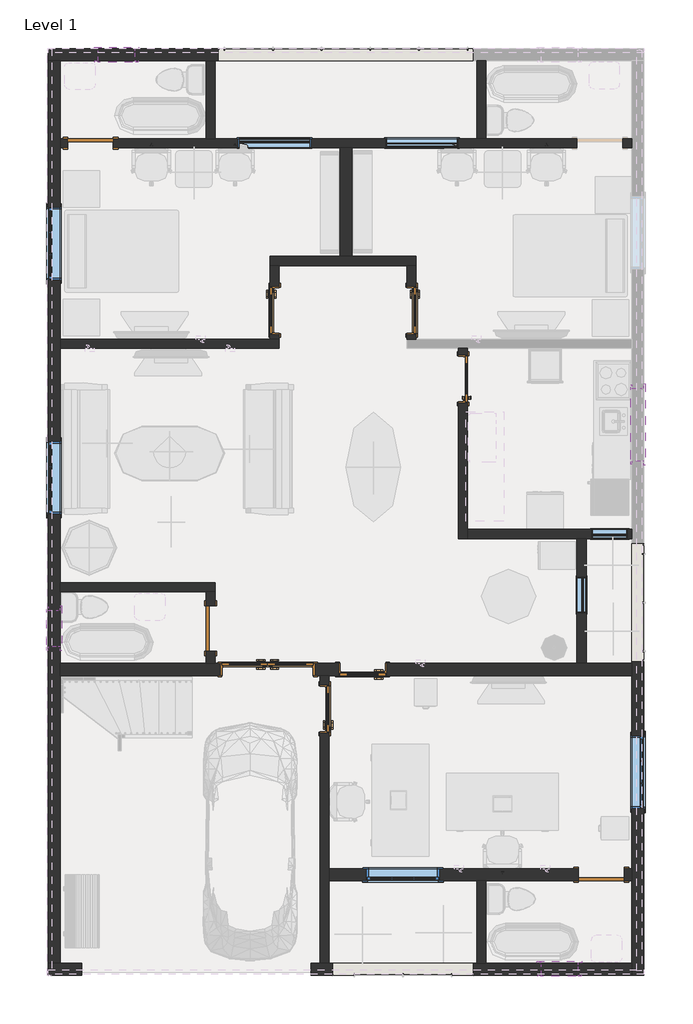
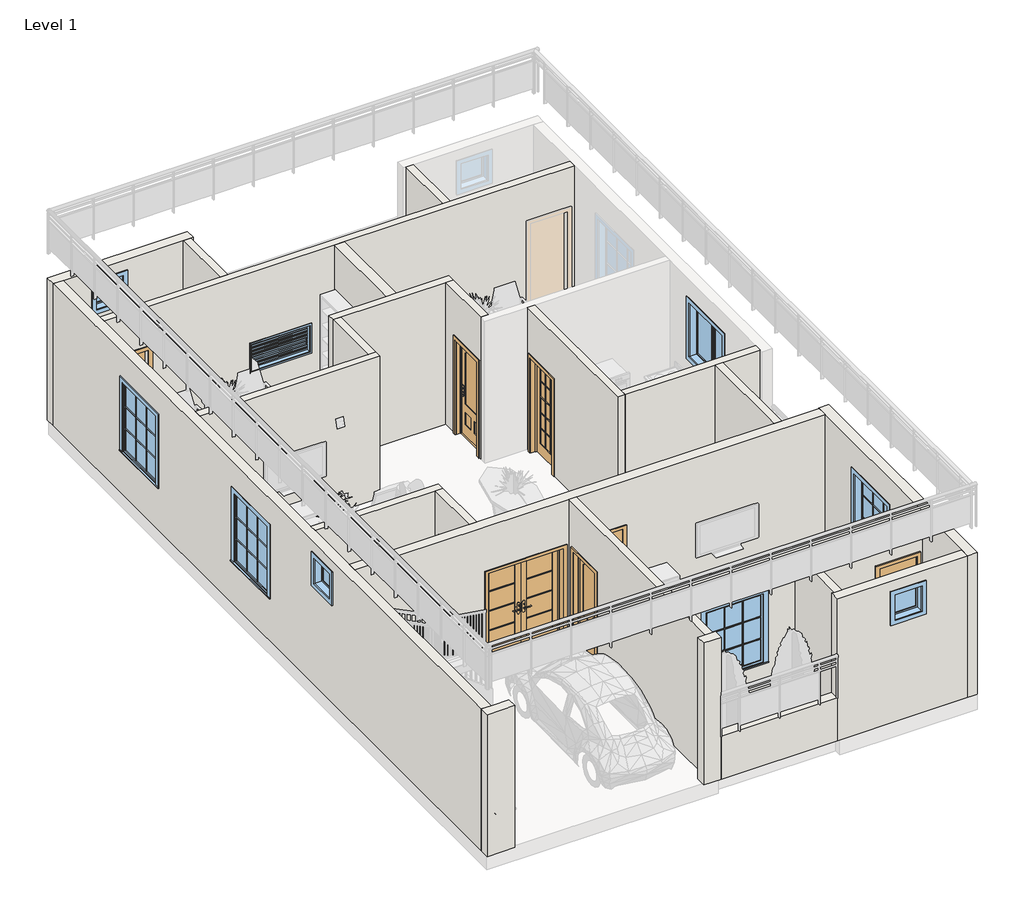
# One storey, part 1 of 5: 26 walls, 12 windows, 9 doors.
"""IFC4 building model written with IfcOpenShell, lengths in millimetres."""

from ifc_helpers import new_model, si_unit, frame, origin, origin_with_axes, place, context, project, spatial, polyline, outline, extrude, faceted_brep, transform, mapped, element, save
from components import door_14b9be53, door_41326d50, door_4b146b56, door_b03bd389, door_a0b5ff2a, door_e2b13fe9, door_4314e8ec, window_cfa1ffdd, window_0862ab64, window_67e7833d, louvers_with_trim_double_60c1390f, window_e41d21a6

model = new_model("IFC4")

# Units and contexts
model_context = context("Model", 3, world=origin())
ifc_project = project(units=[si_unit("LENGTHUNIT", "METRE", prefix="MILLI")], contexts=[model_context])

# Site, building, storey
site = spatial("IfcSite", under=ifc_project)
building = spatial("IfcBuilding", under=site)
storey = spatial("IfcBuildingStorey", under=building, Name="Level 1", Elevation=0.0)

# Doors
placement = place(None, origin())
door_shape = door_14b9be53(model_context)
element("IfcDoor", 1, ObjectType="30\" x 80\"", at=placement, inside=storey, context=model_context, shape_type="MappedRepresentation", body=[
    mapped(door_shape, transform((-2673.2207152, 5044.1691167, 0.0), x_axis=(0.0, -1.0, 0.0), y_axis=(1.0, 0.0, 0.0), z_axis=(0.0, 0.0, 1.0))),
])
element("IfcDoor", 2, ObjectType="30\" x 80\"", at=placement, inside=storey, context=model_context, shape_type="MappedRepresentation", body=[
    mapped(door_shape, transform((-3514.5967824, 11698.9691167, 0.0), x_axis=(0.0, 1.0, 0.0), y_axis=(-1.0, 0.0, 0.0), z_axis=(0.0, 0.0, 1.0))),
])
door_2_shape = door_41326d50(model_context)
element("IfcDoor", 3, ObjectType="30\" x 80\"", at=placement, inside=storey, context=model_context, shape_type="MappedRepresentation", body=[
    mapped(door_2_shape, transform((-2041.3957152, 5701.3941167, 0.0), x_axis=(1.0, 0.0, 0.0), y_axis=(0.0, 1.0, 0.0), z_axis=(0.0, 0.0, 1.0))),
])
door_3_shape = door_4b146b56(model_context)
element("IfcDoor", 4, ObjectType="30\" x 80\"", at=placement, inside=storey, context=model_context, shape_type="MappedRepresentation", body=[
    mapped(door_3_shape, transform((-1222.2467824, 11698.9691167, 0.0), x_axis=(0.0, 1.0, 0.0), y_axis=(-1.0, 0.0, 0.0), z_axis=(0.0, 0.0, 1.0))),
])
door_4_shape = door_b03bd389(model_context)
element("IfcDoor", 5, ObjectType="Door-Exterior-Double-Full Glass-Wood_Clad : 60\" x 80\"", at=placement, inside=storey, context=model_context, shape_type="MappedRepresentation", body=[
    mapped(door_4_shape, transform((-3628.8957152, 5707.7441167, 0.0), x_axis=(1.0, 0.0, 0.0), y_axis=(0.0, 1.0, 0.0), z_axis=(0.0, 0.0, 1.0))),
])
door_5_shape = door_a0b5ff2a(model_context)
element("IfcDoor", 6, ObjectType="Door-Interior-Single-Full Glass-Wood : 30\" x 80\"", at=placement, inside=storey, context=model_context, shape_type="MappedRepresentation", body=[
    mapped(door_5_shape, transform((-361.8207152, 10555.9691167, 0.0), x_axis=(0.0, 1.0, 0.0), y_axis=(-1.0, 0.0, 0.0), z_axis=(0.0, 0.0, 1.0))),
])
door_6_shape = door_e2b13fe9(model_context)
element("IfcDoor", 7, ObjectType="Single-Flush : 30\" x 84\"", at=placement, inside=storey, context=model_context, shape_type="MappedRepresentation", body=[
    mapped(door_6_shape, transform((-6587.9957152, 14492.9691167, 0.0), x_axis=(-1.0, 0.0, 0.0), y_axis=(0.0, -1.0, 0.0), z_axis=(0.0, 0.0, 1.0))),
])
element("IfcDoor", 8, ObjectType="Single-Flush : 30\" x 84\"", at=placement, inside=storey, context=model_context, shape_type="MappedRepresentation", body=[
    mapped(door_6_shape, transform((-4581.3957152, 6390.3691167, 0.0), x_axis=(0.0, -1.0, 0.0), y_axis=(1.0, 0.0, 0.0), z_axis=(0.0, 0.0, 1.0))),
])
door_7_shape = door_4314e8ec(model_context)
element("IfcDoor", 9, ObjectType="Single-Flush : 30\" x 84\"", at=placement, inside=storey, context=model_context, shape_type="MappedRepresentation", body=[
    mapped(door_7_shape, transform((1946.4042848, 2275.5691167, 0.0), x_axis=(1.0, 0.0, 0.0), y_axis=(0.0, 1.0, 0.0), z_axis=(0.0, 0.0, 1.0))),
])

# Walls
element("IfcWall", 10, ObjectType="Generic - 8\"", at=placement, inside=storey, context=model_context, shape_type="Brep", body=[
    faceted_brep([(-7299.1957152, 15864.5691167, 0.0), (-7095.9957152, 15864.5691167, 0.0), (-4657.5957152, 15864.5691167, 0.0), (-4505.1957152, 15864.5691167, 0.0), (-4454.3957152, 15864.5691167, 0.0), (-4454.3957152, 15864.5691167, 914.4), (-4454.3957152, 15864.5691167, 3048.0), (-4505.1957152, 15864.5691167, 3048.0), (-4657.5957152, 15864.5691167, 3048.0), (-7095.9957152, 15864.5691167, 3048.0), (-7299.1957152, 15864.5691167, 3048.0), (-5851.3957152, 15864.5691167, 2768.6), (-5851.3957152, 15864.5691167, 2159.0), (-6460.9957152, 15864.5691167, 2159.0), (-6460.9957152, 15864.5691167, 2768.6), (-7299.1957152, 16067.7691167, 0.0), (-7299.1957152, 16067.7691167, 3048.0), (-4454.3957152, 16067.7691167, 3048.0), (-4454.3957152, 16067.7691167, 914.4), (-4454.3957152, 16067.7691167, 0.0), (-5851.3957152, 16067.7691167, 2768.6), (-6460.9957152, 16067.7691167, 2768.6), (-6460.9957152, 16067.7691167, 2159.0), (-5851.3957152, 16067.7691167, 2159.0)], [[[0, 1, 2, 3, 4, 5, 6, 7, 8, 9, 10], [11, 12, 13, 14]], [[15, 16, 17, 18, 19], [20, 21, 22, 23]], [[4, 3, 2, 1, 0, 15, 19]], [[6, 5, 4, 19, 18, 17]], [[0, 10, 16, 15]], [[10, 9, 8, 7, 6, 17, 16]], [[12, 11, 20, 23]], [[13, 12, 23, 22]], [[14, 13, 22, 21]], [[11, 14, 21, 20]]]),
])
element("IfcWall", 11, ObjectType="Generic - 8\"", at=placement, inside=storey, context=model_context, shape_type="Brep", body=[
    faceted_brep([(2454.4042848, 802.3691167, 0.0), (16.0042848, 802.3691167, 0.0), (-136.3957152, 802.3691167, 0.0), (-187.1957152, 802.3691167, 0.0), (-187.1957152, 802.3691167, 914.4), (-187.1957152, 802.3691167, 3048.0), (-136.3957152, 802.3691167, 3048.0), (16.0042848, 802.3691167, 3048.0), (2454.4042848, 802.3691167, 3048.0), (1552.7042848, 802.3691167, 2768.6), (943.1042848, 802.3691167, 2768.6), (943.1042848, 802.3691167, 2159.0), (1552.7042848, 802.3691167, 2159.0), (2454.4042848, 599.1691167, 0.0), (2454.4042848, 599.1691167, 3048.0), (-187.1957152, 599.1691167, 3048.0), (-187.1957152, 599.1691167, 914.4), (-187.1957152, 599.1691167, 0.0), (1552.7042848, 599.1691167, 2768.6), (1552.7042848, 599.1691167, 2159.0), (943.1042848, 599.1691167, 2159.0), (943.1042848, 599.1691167, 2768.6)], [[[0, 1, 2, 3, 4, 5, 6, 7, 8], [9, 10, 11, 12]], [[13, 14, 15, 16, 17], [18, 19, 20, 21]], [[3, 2, 1, 0, 13, 17]], [[5, 4, 3, 17, 16, 15]], [[0, 8, 14, 13]], [[8, 7, 6, 5, 15, 14]], [[19, 18, 9, 12]], [[20, 19, 12, 11]], [[21, 20, 11, 10]], [[18, 21, 10, 9]]]),
])
element("IfcWall", 12, ObjectType="Generic - 8\"", at=placement, inside=storey, context=model_context, shape_type="Brep", body=[
    faceted_brep([(-7095.9957152, 802.3691167, 0.0), (-7095.9957152, 5602.9691167, 0.0), (-7095.9957152, 5806.1691167, 0.0), (-7095.9957152, 6999.9691167, 0.0), (-7095.9957152, 7152.3691167, 0.0), (-7095.9957152, 11063.9691167, 0.0), (-7095.9957152, 11216.3691167, 0.0), (-7095.9957152, 14416.7691167, 0.0), (-7095.9957152, 14569.1691167, 0.0), (-7095.9957152, 15864.5691167, 0.0), (-7095.9957152, 15864.5691167, 3048.0), (-7095.9957152, 14569.1691167, 3048.0), (-7095.9957152, 14416.7691167, 3048.0), (-7095.9957152, 11216.3691167, 3048.0), (-7095.9957152, 11063.9691167, 3048.0), (-7095.9957152, 7152.3691167, 3048.0), (-7095.9957152, 6999.9691167, 3048.0), (-7095.9957152, 5806.1691167, 3048.0), (-7095.9957152, 5602.9691167, 3048.0), (-7095.9957152, 802.3691167, 3048.0), (-7095.9957152, 9514.5691167, 2438.4), (-7095.9957152, 9514.5691167, 914.4), (-7095.9957152, 8295.3691167, 914.4), (-7095.9957152, 8295.3691167, 2438.4), (-7095.9957152, 13426.1691167, 2438.4), (-7095.9957152, 13426.1691167, 914.4), (-7095.9957152, 12206.9691167, 914.4), (-7095.9957152, 12206.9691167, 2438.4), (-7095.9957152, 6085.5691167, 2768.6), (-7095.9957152, 6695.1691167, 2768.6), (-7095.9957152, 6695.1691167, 2159.0), (-7095.9957152, 6085.5691167, 2159.0), (-7299.1957152, 802.3691167, 0.0), (-7299.1957152, 802.3691167, 3048.0), (-7299.1957152, 15864.5691167, 3048.0), (-7299.1957152, 15864.5691167, 0.0), (-7299.1957152, 9514.5691167, 2438.4), (-7299.1957152, 8295.3691167, 2438.4), (-7299.1957152, 8295.3691167, 914.4), (-7299.1957152, 9514.5691167, 914.4), (-7299.1957152, 13426.1691167, 2438.4), (-7299.1957152, 12206.9691167, 2438.4), (-7299.1957152, 12206.9691167, 914.4), (-7299.1957152, 13426.1691167, 914.4), (-7299.1957152, 6085.5691167, 2768.6), (-7299.1957152, 6085.5691167, 2159.0), (-7299.1957152, 6695.1691167, 2159.0), (-7299.1957152, 6695.1691167, 2768.6)], [[[0, 1, 2, 3, 4, 5, 6, 7, 8, 9, 10, 11, 12, 13, 14, 15, 16, 17, 18, 19], [20, 21, 22, 23], [24, 25, 26, 27], [28, 29, 30, 31]], [[32, 33, 34, 35], [36, 37, 38, 39], [40, 41, 42, 43], [44, 45, 46, 47]], [[9, 8, 7, 6, 5, 4, 3, 2, 1, 0, 32, 35]], [[10, 9, 35, 34]], [[0, 19, 33, 32]], [[19, 18, 17, 16, 15, 14, 13, 12, 11, 10, 34, 33]], [[21, 20, 36, 39]], [[22, 21, 39, 38]], [[23, 22, 38, 37]], [[20, 23, 37, 36]], [[25, 24, 40, 43]], [[26, 25, 43, 42]], [[27, 26, 42, 41]], [[24, 27, 41, 40]], [[45, 44, 28, 31]], [[46, 45, 31, 30]], [[47, 46, 30, 29]], [[44, 47, 29, 28]]]),
])
element("IfcWall", 13, ObjectType="Generic - 8\"", at=placement, inside=storey, context=model_context, shape_type="Brep", body=[
    faceted_brep([(2454.4042848, 5602.9691167, 0.0), (2454.4042848, 5602.9691167, 3048.0), (-2600.1957152, 5602.9691167, 3048.0), (-2752.5957152, 5602.9691167, 3048.0), (-7095.9957152, 5602.9691167, 3048.0), (-7095.9957152, 5602.9691167, 0.0), (-4416.2957152, 5602.9691167, 0.0), (-4416.2957152, 5602.9691167, 2057.4), (-2841.4957152, 5602.9691167, 2057.4), (-2841.4957152, 5602.9691167, 0.0), (-2752.5957152, 5602.9691167, 0.0), (-2600.1957152, 5602.9691167, 0.0), (-2447.7957152, 5602.9691167, 0.0), (-2447.7957152, 5602.9691167, 2057.4), (-1634.9957152, 5602.9691167, 2057.4), (-1634.9957152, 5602.9691167, 0.0), (-7095.9957152, 5806.1691167, 3048.0), (-4657.5957152, 5806.1691167, 3048.0), (-4505.1957152, 5806.1691167, 3048.0), (1540.0042848, 5806.1691167, 3048.0), (1692.4042848, 5806.1691167, 3048.0), (2454.4042848, 5806.1691167, 3048.0), (2454.4042848, 5806.1691167, 0.0), (1692.4042848, 5806.1691167, 0.0), (1540.0042848, 5806.1691167, 0.0), (-1634.9957152, 5806.1691167, 0.0), (-1634.9957152, 5806.1691167, 2057.4), (-2447.7957152, 5806.1691167, 2057.4), (-2447.7957152, 5806.1691167, 0.0), (-2841.4957152, 5806.1691167, 0.0), (-2841.4957152, 5806.1691167, 2057.4), (-4416.2957152, 5806.1691167, 2057.4), (-4416.2957152, 5806.1691167, 0.0), (-4505.1957152, 5806.1691167, 0.0), (-4657.5957152, 5806.1691167, 0.0), (-7095.9957152, 5806.1691167, 0.0)], [[[0, 1, 2, 3, 4, 5, 6, 7, 8, 9, 10, 11, 12, 13, 14, 15]], [[16, 17, 18, 19, 20, 21, 22, 23, 24, 25, 26, 27, 28, 29, 30, 31, 32, 33, 34, 35]], [[5, 35, 34, 33, 32, 6]], [[22, 0, 15, 25, 24, 23]], [[9, 29, 28, 12, 11, 10]], [[1, 0, 22, 21]], [[5, 4, 16, 35]], [[21, 20, 19, 18, 17, 16, 4, 3, 2, 1]], [[8, 30, 29, 9]], [[30, 8, 7, 31]], [[31, 7, 6, 32]], [[14, 26, 25, 15]], [[26, 14, 13, 27]], [[27, 13, 12, 28]]]),
])
element("IfcWall", 14, ObjectType="Generic - 8\"", at=placement, inside=storey, context=model_context, shape_type="Brep", body=[
    faceted_brep([(2327.4042848, 2173.9691167, 2133.6), (2327.4042848, 2173.9691167, 0.0), (2454.4042848, 2173.9691167, 0.0), (2454.4042848, 2173.9691167, 3048.0), (16.0042848, 2173.9691167, 3048.0), (-136.3957152, 2173.9691167, 3048.0), (-2600.1957152, 2173.9691167, 3048.0), (-2600.1957152, 2173.9691167, 0.0), (-136.3957152, 2173.9691167, 0.0), (16.0042848, 2173.9691167, 0.0), (1565.4042848, 2173.9691167, 0.0), (1565.4042848, 2173.9691167, 2133.6), (-1977.8957152, 2173.9691167, 2438.4), (-758.6957152, 2173.9691167, 2438.4), (-758.6957152, 2173.9691167, 914.4), (-1977.8957152, 2173.9691167, 914.4), (2454.4042848, 2377.1691167, 0.0), (2327.4042848, 2377.1691167, 0.0), (2327.4042848, 2377.1691167, 2133.6), (1565.4042848, 2377.1691167, 2133.6), (1565.4042848, 2377.1691167, 0.0), (-2600.1957152, 2377.1691167, 0.0), (-2600.1957152, 2377.1691167, 3048.0), (2454.4042848, 2377.1691167, 3048.0), (-1977.8957152, 2377.1691167, 2438.4), (-1977.8957152, 2377.1691167, 914.4), (-758.6957152, 2377.1691167, 914.4), (-758.6957152, 2377.1691167, 2438.4)], [[[0, 1, 2, 3, 4, 5, 6, 7, 8, 9, 10, 11], [12, 13, 14, 15]], [[16, 17, 18, 19, 20, 21, 22, 23], [24, 25, 26, 27]], [[2, 1, 17, 16]], [[10, 9, 8, 7, 21, 20]], [[3, 2, 16, 23]], [[7, 6, 22, 21]], [[6, 5, 4, 3, 23, 22]], [[18, 17, 1, 0]], [[19, 18, 0, 11]], [[20, 19, 11, 10]], [[25, 24, 12, 15]], [[26, 25, 15, 14]], [[27, 26, 14, 13]], [[24, 27, 13, 12]]]),
])
element("IfcWall", 15, ObjectType="Generic - 8\"", at=placement, inside=storey, context=model_context, shape_type="SweptSolid", body=[
    extrude(outline(polyline([(-2422.3957152, 12601.2939646), (-2422.3957152, 14416.7691167), (-2219.1957152, 14416.7691167), (-2219.1957152, 12601.2939646), (-2422.3957152, 12601.2939646)])), origin_with_axes(), (0.0, 0.0, 1.0), 3048.0),
])
element("IfcWall", 16, ObjectType="Generic - 8\"", at=placement, inside=storey, context=model_context, shape_type="SweptSolid", body=[
    extrude(outline(polyline([(-187.1957152, 15864.5691167), (-4454.3957152, 15864.5691167), (-4454.3957152, 16067.7691167), (-187.1957152, 16067.7691167), (-187.1957152, 15864.5691167)])), origin_with_axes(), (0.0, 0.0, 1.0), 914.4),
])
element("IfcWall", 17, ObjectType="Generic - 8\"", at=placement, inside=storey, context=model_context, shape_type="SweptSolid", body=[
    extrude(outline(polyline([(2454.4042848, 5831.5691167), (2454.4042848, 7812.7691167), (2657.6042848, 7812.7691167), (2657.6042848, 5831.5691167), (2454.4042848, 5831.5691167)])), origin_with_axes(), (0.0, 0.0, 1.0), 914.4),
])
element("IfcWall", 18, ObjectType="Generic - 8\"", at=placement, inside=storey, context=model_context, shape_type="Brep", body=[
    faceted_brep([(2454.4042848, 5831.5691167, 0.0), (2454.4042848, 5806.1691167, 0.0), (2454.4042848, 5602.9691167, 0.0), (2454.4042848, 2377.1691167, 0.0), (2454.4042848, 2173.9691167, 0.0), (2454.4042848, 802.3691167, 0.0), (2454.4042848, 599.1691167, 0.0), (2454.4042848, 599.1691167, 3048.0), (2454.4042848, 802.3691167, 3048.0), (2454.4042848, 2173.9691167, 3048.0), (2454.4042848, 2377.1691167, 3048.0), (2454.4042848, 5602.9691167, 3048.0), (2454.4042848, 5806.1691167, 3048.0), (2454.4042848, 5831.5691167, 3048.0), (2454.4042848, 5831.5691167, 914.4), (2454.4042848, 3380.4691167, 2438.4), (2454.4042848, 3380.4691167, 914.4), (2454.4042848, 4599.6691167, 914.4), (2454.4042848, 4599.6691167, 2438.4), (2657.6042848, 5831.5691167, 0.0), (2657.6042848, 5831.5691167, 914.4), (2657.6042848, 5831.5691167, 3048.0), (2657.6042848, 599.1691167, 3048.0), (2657.6042848, 599.1691167, 0.0), (2657.6042848, 3380.4691167, 2438.4), (2657.6042848, 4599.6691167, 2438.4), (2657.6042848, 4599.6691167, 914.4), (2657.6042848, 3380.4691167, 914.4)], [[[0, 1, 2, 3, 4, 5, 6, 7, 8, 9, 10, 11, 12, 13, 14], [15, 16, 17, 18]], [[19, 20, 21, 22, 23], [24, 25, 26, 27]], [[6, 5, 4, 3, 2, 1, 0, 19, 23]], [[0, 14, 13, 21, 20, 19]], [[7, 6, 23, 22]], [[13, 12, 11, 10, 9, 8, 7, 22, 21]], [[16, 15, 24, 27]], [[17, 16, 27, 26]], [[18, 17, 26, 25]], [[15, 18, 25, 24]]]),
])
element("IfcWall", 19, ObjectType="Generic - 8\"", at=placement, inside=storey, context=model_context, shape_type="Brep", body=[
    faceted_brep([(-6740.3957152, 802.3691167, 0.0), (-7095.9957152, 802.3691167, 0.0), (-7299.1957152, 802.3691167, 0.0), (-7299.1957152, 802.3691167, 3048.0), (-7095.9957152, 802.3691167, 3048.0), (-6740.3957152, 802.3691167, 3048.0), (-6740.3957152, 599.1691167, 0.0), (-6740.3957152, 599.1691167, 3048.0), (-7299.1957152, 599.1691167, 3048.0), (-7299.1957152, 599.1691167, 0.0)], [[[0, 1, 2, 3, 4, 5]], [[6, 7, 8, 9]], [[2, 1, 0, 6, 9]], [[0, 5, 7, 6]], [[3, 2, 9, 8]], [[5, 4, 3, 8, 7]]]),
])
element("IfcWall", 20, ObjectType="Generic - 8\"", at=placement, inside=storey, context=model_context, shape_type="Brep", body=[
    faceted_brep([(-2549.3957152, 802.3691167, 0.0), (-2600.1957152, 802.3691167, 0.0), (-2752.5957152, 802.3691167, 0.0), (-2904.9957152, 802.3691167, 0.0), (-2904.9957152, 802.3691167, 3048.0), (-2752.5957152, 802.3691167, 3048.0), (-2600.1957152, 802.3691167, 3048.0), (-2549.3957152, 802.3691167, 3048.0), (-2549.3957152, 802.3691167, 914.4), (-2549.3957152, 599.1691167, 0.0), (-2549.3957152, 599.1691167, 914.4), (-2549.3957152, 599.1691167, 3048.0), (-2904.9957152, 599.1691167, 3048.0), (-2904.9957152, 599.1691167, 0.0)], [[[0, 1, 2, 3, 4, 5, 6, 7, 8]], [[9, 10, 11, 12, 13]], [[3, 2, 1, 0, 9, 13]], [[4, 3, 13, 12]], [[0, 8, 7, 11, 10, 9]], [[7, 6, 5, 4, 12, 11]]]),
])
element("IfcWall", 21, ObjectType="Generic - 8\"", at=placement, inside=storey, context=model_context, shape_type="SweptSolid", body=[
    extrude(outline(polyline([(-2549.3957152, 802.3691167), (-187.1957152, 802.3691167), (-187.1957152, 599.1691167), (-2549.3957152, 599.1691167), (-2549.3957152, 802.3691167)])), origin_with_axes(), (0.0, 0.0, 1.0), 914.4),
])
element("IfcWall", 22, ObjectType="inner wall", at=placement, inside=storey, context=model_context, shape_type="Brep", body=[
    faceted_brep([(2302.0042848, 14416.7691167, 2133.6), (2302.0042848, 14416.7691167, 0.0), (2454.4042848, 14416.7691167, 0.0), (2454.4042848, 14416.7691167, 3048.0), (-2219.1957152, 14416.7691167, 3048.0), (-2422.3957152, 14416.7691167, 3048.0), (-7095.9957152, 14416.7691167, 3048.0), (-7095.9957152, 14416.7691167, 0.0), (-6968.9957152, 14416.7691167, 0.0), (-6968.9957152, 14416.7691167, 2133.6), (-6206.9957152, 14416.7691167, 2133.6), (-6206.9957152, 14416.7691167, 0.0), (-2422.3957152, 14416.7691167, 0.0), (-2219.1957152, 14416.7691167, 0.0), (1540.0042848, 14416.7691167, 0.0), (1540.0042848, 14416.7691167, 2133.6), (-2904.9957152, 14416.7691167, 1524.0), (-2904.9957152, 14416.7691167, 914.4), (-4124.1957152, 14416.7691167, 914.4), (-4124.1957152, 14416.7691167, 1524.0), (-1660.3957152, 14416.7691167, 1524.0), (-441.1957152, 14416.7691167, 1524.0), (-441.1957152, 14416.7691167, 914.4), (-1660.3957152, 14416.7691167, 914.4), (2454.4042848, 14569.1691167, 0.0), (2302.0042848, 14569.1691167, 0.0), (2302.0042848, 14569.1691167, 2133.6), (1540.0042848, 14569.1691167, 2133.6), (1540.0042848, 14569.1691167, 0.0), (16.0042848, 14569.1691167, 0.0), (-136.3957152, 14569.1691167, 0.0), (-4505.1957152, 14569.1691167, 0.0), (-4657.5957152, 14569.1691167, 0.0), (-6206.9957152, 14569.1691167, 0.0), (-6206.9957152, 14569.1691167, 2133.6), (-6968.9957152, 14569.1691167, 2133.6), (-6968.9957152, 14569.1691167, 0.0), (-7095.9957152, 14569.1691167, 0.0), (-7095.9957152, 14569.1691167, 3048.0), (-4657.5957152, 14569.1691167, 3048.0), (-4505.1957152, 14569.1691167, 3048.0), (-136.3957152, 14569.1691167, 3048.0), (16.0042848, 14569.1691167, 3048.0), (2454.4042848, 14569.1691167, 3048.0), (-2904.9957152, 14569.1691167, 1524.0), (-4124.1957152, 14569.1691167, 1524.0), (-4124.1957152, 14569.1691167, 914.4), (-2904.9957152, 14569.1691167, 914.4), (-1660.3957152, 14569.1691167, 1524.0), (-1660.3957152, 14569.1691167, 914.4), (-441.1957152, 14569.1691167, 914.4), (-441.1957152, 14569.1691167, 1524.0)], [[[0, 1, 2, 3, 4, 5, 6, 7, 8, 9, 10, 11, 12, 13, 14, 15], [16, 17, 18, 19], [20, 21, 22, 23]], [[24, 25, 26, 27, 28, 29, 30, 31, 32, 33, 34, 35, 36, 37, 38, 39, 40, 41, 42, 43], [44, 45, 46, 47], [48, 49, 50, 51]], [[37, 36, 8, 7]], [[2, 1, 25, 24]], [[14, 13, 12, 11, 33, 32, 31, 30, 29, 28]], [[3, 2, 24, 43]], [[7, 6, 38, 37]], [[6, 5, 4, 3, 43, 42, 41, 40, 39, 38]], [[9, 8, 36, 35]], [[10, 9, 35, 34]], [[11, 10, 34, 33]], [[26, 25, 1, 0]], [[27, 26, 0, 15]], [[28, 27, 15, 14]], [[17, 16, 44, 47]], [[18, 17, 47, 46]], [[19, 18, 46, 45]], [[16, 19, 45, 44]], [[49, 48, 20, 23]], [[50, 49, 23, 22]], [[51, 50, 22, 21]], [[48, 51, 21, 20]]]),
])
element("IfcWall", 23, ObjectType="inner wall", at=placement, inside=storey, context=model_context, shape_type="SweptSolid", body=[
    extrude(outline(polyline([(-4657.5957152, 14569.1691167), (-4657.5957152, 15864.5691167), (-4505.1957152, 15864.5691167), (-4505.1957152, 14569.1691167), (-4657.5957152, 14569.1691167)])), origin_with_axes(), (0.0, 0.0, 1.0), 3048.0),
])
element("IfcWall", 24, ObjectType="inner wall", at=placement, inside=storey, context=model_context, shape_type="SweptSolid", body=[
    extrude(outline(polyline([(-136.3957152, 14569.1691167), (-136.3957152, 15864.5691167), (16.0042848, 15864.5691167), (16.0042848, 14569.1691167), (-136.3957152, 14569.1691167)])), origin_with_axes(), (0.0, 0.0, 1.0), 3048.0),
])
element("IfcWall", 25, ObjectType="inner wall", at=placement, inside=storey, context=model_context, shape_type="Brep", body=[
    faceted_brep([(-7095.9957152, 11063.9691167, 0.0), (-3435.2217824, 11063.9691167, 0.0), (-3435.2217824, 11063.9691167, 3048.0), (-7095.9957152, 11063.9691167, 3048.0), (-7095.9957152, 11216.3691167, 0.0), (-7095.9957152, 11216.3691167, 3048.0), (-3587.6217824, 11216.3691167, 3048.0), (-3435.2217824, 11216.3691167, 3048.0), (-3435.2217824, 11216.3691167, 0.0), (-3587.6217824, 11216.3691167, 0.0)], [[[0, 1, 2, 3]], [[4, 5, 6, 7, 8, 9]], [[1, 0, 4, 9, 8]], [[0, 3, 5, 4]], [[2, 1, 8, 7]], [[3, 2, 7, 6, 5]]]),
])
element("IfcWall", 26, ObjectType="inner wall", at=placement, inside=storey, context=model_context, shape_type="Brep", body=[
    faceted_brep([(-2752.5957152, 802.3691167, 0.0), (-2752.5957152, 802.3691167, 3048.0), (-2752.5957152, 3036.4892317, 3048.0), (-2752.5957152, 5602.9691167, 3048.0), (-2752.5957152, 5602.9691167, 0.0), (-2752.5957152, 5450.5691167, 0.0), (-2752.5957152, 5450.5691167, 2057.4), (-2752.5957152, 4637.7691167, 2057.4), (-2752.5957152, 4637.7691167, 0.0), (-2600.1957152, 5602.9691167, 3048.0), (-2600.1957152, 2377.1691167, 3048.0), (-2600.1957152, 2173.9691167, 3048.0), (-2600.1957152, 802.3691167, 3048.0), (-2600.1957152, 802.3691167, 0.0), (-2600.1957152, 2173.9691167, 0.0), (-2600.1957152, 2377.1691167, 0.0), (-2600.1957152, 4637.7691167, 0.0), (-2600.1957152, 4637.7691167, 2057.4), (-2600.1957152, 5450.5691167, 2057.4), (-2600.1957152, 5450.5691167, 0.0), (-2600.1957152, 5602.9691167, 0.0)], [[[0, 1, 2, 3, 4, 5, 6, 7, 8]], [[9, 10, 11, 12, 13, 14, 15, 16, 17, 18, 19, 20]], [[4, 20, 19, 5]], [[13, 0, 8, 16, 15, 14]], [[1, 0, 13, 12]], [[4, 3, 9, 20]], [[12, 11, 10, 9, 3, 2, 1]], [[7, 17, 16, 8]], [[17, 7, 6, 18]], [[18, 6, 5, 19]]]),
])
element("IfcWall", 27, ObjectType="inner wall", at=placement, inside=storey, context=model_context, shape_type="SweptSolid", body=[
    extrude(outline(polyline([(-136.3957152, 802.3691167), (-136.3957152, 2173.9691167), (16.0042848, 2173.9691167), (16.0042848, 802.3691167), (-136.3957152, 802.3691167)])), origin_with_axes(), (0.0, 0.0, 1.0), 3048.0),
])
element("IfcWall", 28, ObjectType="inner wall", at=placement, inside=storey, context=model_context, shape_type="Brep", body=[
    faceted_brep([(-3587.6217824, 12448.8939646, 0.0), (-3435.2217824, 12448.8939646, 0.0), (-1301.6217824, 12448.8939646, 0.0), (-1149.2217824, 12448.8939646, 0.0), (-1149.2217824, 12448.8939646, 3048.0), (-1301.6217824, 12448.8939646, 3048.0), (-3435.2217824, 12448.8939646, 3048.0), (-3587.6217824, 12448.8939646, 3048.0), (-3587.6217824, 12601.2939646, 0.0), (-3587.6217824, 12601.2939646, 3048.0), (-2422.3957152, 12601.2939646, 3048.0), (-2219.1957152, 12601.2939646, 3048.0), (-1149.2217824, 12601.2939646, 3048.0), (-1149.2217824, 12601.2939646, 0.0), (-2219.1957152, 12601.2939646, 0.0), (-2422.3957152, 12601.2939646, 0.0)], [[[0, 1, 2, 3, 4, 5, 6, 7]], [[8, 9, 10, 11, 12, 13, 14, 15]], [[3, 2, 1, 0, 8, 15, 14, 13]], [[4, 3, 13, 12]], [[0, 7, 9, 8]], [[7, 6, 5, 4, 12, 11, 10, 9]]]),
])
element("IfcWall", 29, ObjectType="inner wall", at=placement, inside=storey, context=model_context, shape_type="SweptSolid", body=[
    extrude(outline(polyline([(12448.8939646, 3048.0), (12448.8939646, 0.0), (12105.3691167, 0.0), (12105.3691167, 2057.4), (11292.5691167, 2057.4), (11292.5691167, 0.0), (11216.3691167, 0.0), (11216.3691167, 3048.0), (12448.8939646, 3048.0)])), frame((-1301.6217824, 0.0, 0.0), z_axis=(1.0, 0.0, 0.0), x_axis=(0.0, 1.0, 0.0)), (0.0, 0.0, 1.0), 152.4),
])
element("IfcWall", 30, ObjectType="inner wall", at=placement, inside=storey, context=model_context, shape_type="SweptSolid", body=[
    extrude(outline(polyline([(12448.8939646, 3048.0), (12448.8939646, 0.0), (12105.3691167, 0.0), (12105.3691167, 2057.4), (11292.5691167, 2057.4), (11292.5691167, 0.0), (11216.3691167, 0.0), (11216.3691167, 3048.0), (12448.8939646, 3048.0)])), frame((-3587.6217824, 0.0, 0.0), z_axis=(1.0, 0.0, 0.0), x_axis=(0.0, 1.0, 0.0)), (0.0, 0.0, 1.0), 152.4),
])
element("IfcWall", 31, ObjectType="inner wall", at=placement, inside=storey, context=model_context, shape_type="Brep", body=[
    faceted_brep([(-441.1957152, 11063.9691167, 3048.0), (-441.1957152, 11063.9691167, 0.0), (-441.1957152, 10962.3691167, 0.0), (-441.1957152, 10962.3691167, 2057.4), (-441.1957152, 10149.5691167, 2057.4), (-441.1957152, 10149.5691167, 0.0), (-441.1957152, 7888.9691167, 0.0), (-441.1957152, 7888.9691167, 3048.0), (-288.7957152, 11063.9691167, 0.0), (-288.7957152, 11063.9691167, 3048.0), (-288.7957152, 8041.3691167, 3048.0), (-288.7957152, 7888.9691167, 3048.0), (-288.7957152, 7888.9691167, 0.0), (-288.7957152, 8041.3691167, 0.0), (-288.7957152, 10149.5691167, 0.0), (-288.7957152, 10149.5691167, 2057.4), (-288.7957152, 10962.3691167, 2057.4), (-288.7957152, 10962.3691167, 0.0)], [[[0, 1, 2, 3, 4, 5, 6, 7]], [[8, 9, 10, 11, 12, 13, 14, 15, 16, 17]], [[1, 8, 17, 2]], [[12, 6, 5, 14, 13]], [[1, 0, 9, 8]], [[7, 6, 12, 11]], [[0, 7, 11, 10, 9]], [[16, 3, 2, 17]], [[3, 16, 15, 4]], [[4, 15, 14, 5]]]),
])
element("IfcWall", 32, ObjectType="inner wall", at=placement, inside=storey, context=model_context, shape_type="Brep", body=[
    faceted_brep([(2454.4042848, 8041.3691167, 0.0), (-288.7957152, 8041.3691167, 0.0), (-288.7957152, 8041.3691167, 3048.0), (2454.4042848, 8041.3691167, 3048.0), (1781.3042848, 8041.3691167, 1524.0), (1781.3042848, 8041.3691167, 914.4), (2390.9042848, 8041.3691167, 914.4), (2390.9042848, 8041.3691167, 1524.0), (-288.7957152, 7888.9691167, 0.0), (1540.0042848, 7888.9691167, 0.0), (1692.4042848, 7888.9691167, 0.0), (2454.4042848, 7888.9691167, 0.0), (2454.4042848, 7888.9691167, 3048.0), (1692.4042848, 7888.9691167, 3048.0), (1540.0042848, 7888.9691167, 3048.0), (-288.7957152, 7888.9691167, 3048.0), (1781.3042848, 7888.9691167, 914.4), (1781.3042848, 7888.9691167, 1524.0), (2390.9042848, 7888.9691167, 1524.0), (2390.9042848, 7888.9691167, 914.4)], [[[0, 1, 2, 3], [4, 5, 6, 7]], [[8, 9, 10, 11, 12, 13, 14, 15], [16, 17, 18, 19]], [[1, 0, 11, 10, 9, 8]], [[0, 3, 12, 11]], [[2, 1, 8, 15]], [[3, 2, 15, 14, 13, 12]], [[4, 17, 16, 5]], [[5, 16, 19, 6]], [[17, 4, 7, 18]], [[18, 7, 6, 19]]]),
])
element("IfcWall", 33, ObjectType="inner wall", at=placement, inside=storey, context=model_context, shape_type="SweptSolid", body=[
    extrude(outline(polyline([(7888.9691167, 0.0), (5806.1691167, 0.0), (5806.1691167, 3048.0), (7888.9691167, 3048.0), (7888.9691167, 0.0)]), holes=[polyline([(6644.3691167, 1524.0), (6644.3691167, 914.4), (7253.9691167, 914.4), (7253.9691167, 1524.0), (6644.3691167, 1524.0)])]), frame((1540.0042848, 0.0, 0.0), z_axis=(1.0, 0.0, 0.0), x_axis=(0.0, 1.0, 0.0)), (0.0, 0.0, 1.0), 152.4),
])
element("IfcWall", 34, ObjectType="inner wall", at=placement, inside=storey, context=model_context, shape_type="Brep", body=[
    faceted_brep([(-7095.9957152, 6999.9691167, 0.0), (-4657.5957152, 6999.9691167, 0.0), (-4505.1957152, 6999.9691167, 0.0), (-4505.1957152, 6999.9691167, 3048.0), (-4657.5957152, 6999.9691167, 3048.0), (-7095.9957152, 6999.9691167, 3048.0), (-7095.9957152, 7152.3691167, 0.0), (-7095.9957152, 7152.3691167, 3048.0), (-4505.1957152, 7152.3691167, 3048.0), (-4505.1957152, 7152.3691167, 0.0)], [[[0, 1, 2, 3, 4, 5]], [[6, 7, 8, 9]], [[2, 1, 0, 6, 9]], [[0, 5, 7, 6]], [[3, 2, 9, 8]], [[5, 4, 3, 8, 7]]]),
])
element("IfcWall", 35, ObjectType="inner wall", at=placement, inside=storey, context=model_context, shape_type="SweptSolid", body=[
    extrude(outline(polyline([(6009.3691167, 2133.6), (6009.3691167, 0.0), (5806.1691167, 0.0), (5806.1691167, 3048.0), (6999.9691167, 3048.0), (6999.9691167, 0.0), (6771.3691167, 0.0), (6771.3691167, 2133.6), (6009.3691167, 2133.6)])), frame((-4657.5957152, 0.0, 0.0), z_axis=(1.0, 0.0, 0.0), x_axis=(0.0, 1.0, 0.0)), (0.0, 0.0, 1.0), 152.4),
])

# Windows
window_shape = window_cfa1ffdd(model_context)
element("IfcWindow", 36, ObjectType="Casement 3x3 with Trim : 48\" x 60\"", at=placement, inside=storey, context=model_context, shape_type="MappedRepresentation", body=[
    mapped(window_shape, transform((-1368.2957152, 2275.5691167, 304.8), x_axis=(-1.0, 0.0, 0.0), y_axis=(0.0, -1.0, 0.0), z_axis=(0.0, 0.0, 1.0))),
])
element("IfcWindow", 37, ObjectType="Casement 3x3 with Trim : 48\" x 60\"", at=placement, inside=storey, context=model_context, shape_type="MappedRepresentation", body=[
    mapped(window_shape, transform((2556.0042848, 3990.0691167, 304.8), x_axis=(0.0, -1.0, 0.0), y_axis=(1.0, 0.0, 0.0), z_axis=(0.0, 0.0, 1.0))),
])
element("IfcWindow", 38, ObjectType="Casement 3x3 with Trim : 48\" x 60\"", at=placement, inside=storey, context=model_context, shape_type="MappedRepresentation", body=[
    mapped(window_shape, transform((-7197.5957152, 8904.9691167, 304.8), x_axis=(0.0, 1.0, 0.0), y_axis=(-1.0, 0.0, 0.0), z_axis=(0.0, 0.0, 1.0))),
])
element("IfcWindow", 39, ObjectType="Casement 3x3 with Trim : 48\" x 60\"", at=placement, inside=storey, context=model_context, shape_type="MappedRepresentation", body=[
    mapped(window_shape, transform((-7197.5957152, 12816.5691167, 304.8), x_axis=(0.0, 1.0, 0.0), y_axis=(-1.0, 0.0, 0.0), z_axis=(0.0, 0.0, 1.0))),
])
window_2_shape = window_0862ab64(model_context)
element("IfcWindow", 40, ObjectType="Casement Dbl with Trim : 48\" x 48\"", at=placement, inside=storey, context=model_context, shape_type="MappedRepresentation", body=[
    mapped(window_2_shape, transform((2536.9542848, 9793.9691167, 457.2), x_axis=(0.0, -1.0, 0.0), y_axis=(1.0, 0.0, 0.0), z_axis=(0.0, 0.0, 1.0))),
])
window_3_shape = window_67e7833d(model_context)
element("IfcWindow", 41, ObjectType="Louvers with Trim : 24\" x 24\"", at=placement, inside=storey, context=model_context, shape_type="MappedRepresentation", body=[
    mapped(window_3_shape, transform((-3514.5957152, 14499.3191167, 0.0), x_axis=(1.0, 0.0, 0.0), y_axis=(0.0, 1.0, 0.0), z_axis=(0.0, 0.0, 1.0))),
])
element("IfcWindow", 42, ObjectType="Louvers with Trim : 24\" x 24\"", at=placement, inside=storey, context=model_context, shape_type="MappedRepresentation", body=[
    mapped(window_3_shape, transform((-1050.7957152, 14486.6191167, 0.0), x_axis=(-1.0, 0.0, 0.0), y_axis=(0.0, -1.0, 0.0), z_axis=(0.0, 0.0, 1.0))),
])
louvers_with_trim_double_shape = louvers_with_trim_double_60c1390f(model_context)
element("IfcWindow", 43, ObjectType="Louvers with Trim : DOUBLE", at=placement, inside=storey, context=model_context, shape_type="MappedRepresentation", body=[
    mapped(louvers_with_trim_double_shape, transform((2086.1042848, 7958.8191167, 0.0), x_axis=(-1.0, 0.0, 0.0), y_axis=(0.0, -1.0, 0.0), z_axis=(0.0, 0.0, 1.0))),
])
element("IfcWindow", 44, ObjectType="Louvers with Trim : DOUBLE", at=placement, inside=storey, context=model_context, shape_type="MappedRepresentation", body=[
    mapped(louvers_with_trim_double_shape, transform((1622.5542848, 6949.1691167, 0.0), x_axis=(0.0, -1.0, 0.0), y_axis=(1.0, 0.0, 0.0), z_axis=(0.0, 0.0, 1.0))),
])
window_4_shape = window_e41d21a6(model_context)
element("IfcWindow", 45, ObjectType="Transom with Trim : 24\" x 24\"", at=placement, inside=storey, context=model_context, shape_type="MappedRepresentation", body=[
    mapped(window_4_shape, transform((-6118.0957152, 15966.1691167, 0.0), x_axis=(1.0, 0.0, 0.0), y_axis=(0.0, 1.0, 0.0), z_axis=(0.0, 0.0, 1.0))),
])
element("IfcWindow", 46, ObjectType="Transom with Trim : 24\" x 24\"", at=placement, inside=storey, context=model_context, shape_type="MappedRepresentation", body=[
    mapped(window_4_shape, transform((-7197.5957152, 6352.2691167, 0.0), x_axis=(0.0, -1.0, 0.0), y_axis=(1.0, 0.0, 0.0), z_axis=(0.0, 0.0, 1.0))),
])
element("IfcWindow", 47, ObjectType="Transom with Trim : 24\" x 24\"", at=placement, inside=storey, context=model_context, shape_type="MappedRepresentation", body=[
    mapped(window_4_shape, transform((1286.0042848, 700.7691167, 0.0), x_axis=(1.0, 0.0, 0.0), y_axis=(0.0, 1.0, 0.0), z_axis=(0.0, 0.0, 1.0))),
])

save(model, "model.ifc")

# Revit data of these elements
# Type "30\" x 80\""
#   Type Mark = "9"
#   Assembly Code = "B2030100"
#   Analytic Construction = "French door, wood frame with single glass"
#   Threshold Offset [instance default] = 0' - 0 1/2"
#   Thickness = 0' - 1 3/8"
#   Thermal Resistance (R) = 1.0696 (h·ft²·°F)/BTU
#   Swing Angle [instance default] = 90.00°
#   Stiles = 0' - 4 3/4"
#   Rough Width = 2' - 8"
#   Rough Height = 6' - 9"
#   Radius = 1' - 1.00625"
#   Lock Rail = 0' - 7 1/8"
#   Height = 6' - 8"
#   Width = 2' - 6"
#   Heat Transfer Coefficient (U) = 0.9350 BTU/(h·ft²·°F)
#   Door Offset [instance default] = 0' - 0"
#   Bottom Rail = 0' - 9 1/2"
#   Threshold [instance default] = yes
#   Function = 1
#   Exterior Trim [instance default] = yes
#   Trim Material = Cherry
#   Threshold Material = Cherry
#   Panel Material = Cherry
#   Glazing = Glass
#   Frame Material = Cherry
#   Door Handle Material = Aluminum
#   Visual Light Transmittance = 0
#   Solar Heat Gain Coefficient = 0
#   Wall Closure = (empty or 0)
#   Construction Type = (empty or 0)
# Type "Door-Exterior-Double-Full Glass-Wood_Clad : 60\" x 80\""
#   Type Mark = "8"
#   Assembly Code = "B2030100"
#   Analytic Construction = "French door, wood frame with double glass"
#   Top Rail = 0' - 4 11/16"
#   Threshold Offset [instance default] = 0' - 0 1/2"
#   Thickness = 0' - 1 3/8"
#   Thermal Resistance (R) = 1.9158 (h·ft²·°F)/BTU
#   Swing Angle [instance default] = 90.00°
#   Stiles = 0' - 4 3/4"
#   Rough Width = 5' - 2"
#   Rough Height = 6' - 9"
#   Panel Width = 2' - 6"
#   Door Offset [instance default] = 0' - 0"
#   Height = 6' - 8"
#   Width = 5' - 0"
#   Heat Transfer Coefficient (U) = 0.5220 BTU/(h·ft²·°F)
#   Bottom Rail = 0' - 9 1/8"
#   Exterior Trim [instance default] = yes
#   Threshold [instance default] = yes
#   Show Grill [instance default] = yes
#   Function = 1
#   Trim Material = Cherry
#   Threshold Material = Cherry
#   Panel Material = Cherry
#   Glazing = Glass
#   Frame Material = Cherry
#   Door Handle Material = Aluminum
#   Visual Light Transmittance = 0
#   Solar Heat Gain Coefficient = 0
#   Wall Closure = (empty or 0)
#   Construction Type = (empty or 0)
# Type "Door-Interior-Single-Full Glass-Wood : 30\" x 80\""
#   Type Mark = "10"
#   Assembly Code = "C1020300"
#   Analytic Construction = "Wood frame with single clear glass"
#   Top Rail = 0' - 4 11/16"
#   Thickness = 0' - 1 3/8"
#   Thermal Resistance (R) = 1.0102 (h·ft²·°F)/BTU
#   Swing Angle [instance default] = 90.00°
#   Stiles = 0' - 4 3/4"
#   Rough Width = 2' - 8"
#   Rough Height = 6' - 9"
#   Height = 6' - 8"
#   Width = 2' - 6"
#   Heat Transfer Coefficient (U) = 0.9900 BTU/(h·ft²·°F)
#   Bottom Rail = 0' - 9 1/8"
#   Show Grill [instance default] = yes
#   Trim Material = Cherry
#   Panel Material = Cherry
#   Frame Material = Cherry
#   Door Handle Material = Aluminum
#   Visual Light Transmittance = 0
#   Solar Heat Gain Coefficient = 0
#   Wall Closure = (empty or 0)
#   Function = (empty or 0)
# Type "Single-Flush : 30\" x 84\""
#   Type Mark = "4"
#   Construction Type Id = "MDOOR"
#   Assembly Code = "C1020"
#   Analytic Construction = "Metal"
#   Thickness = 0' - 2"
#   Heat Transfer Coefficient (U) = 0.651978 BTU/(h·ft²·°F)
#   Height = 7' - 0"
#   Trim Projection Ext = 0' - 1"
#   Trim Projection Int = 0' - 1"
#   Trim Width = 0' - 3"
#   Width = 2' - 6"
#   Define Thermal Properties by = 1
#   Door Material = Door - Panel
#   Frame Material = Door - Frame
#   Visual Light Transmittance = 0
#   Solar Heat Gain Coefficient = 0
#   Function = (empty or 0)
#   Wall Closure = (empty or 0)
# Type "Generic - 8\""
#   Assembly Code = "B2010"
#   Layers, outside or top first: 0' - 8" "Brick, Common" (function 1)
# Type "inner wall"
#   Assembly Code = "B2010"
#   Layers, outside or top first: 0' - 6" "Brick, Soldier Course" (function 1)
# Type "Casement 3x3 with Trim : 48\" x 60\""
#   Type Mark = "11"
#   Construction Type Id = "GSP4R"
#   Assembly Code = "B2020100"
#   Analytic Construction = "1/8 in Pilkington single glazing"
#   Visual Light Transmittance = 0.9
#   Solar Heat Gain Coefficient = 0.78
#   Heat Transfer Coefficient (U) = 0.6496 BTU/(h·ft²·°F)
#   Height = 5' - 0"
#   Default Sill Height = 2' - 0"
#   Trim Projection - Ext. = 0' - 0 1/2"
#   Trim Projection - Int. = 0' - 0 3/4"
#   Trim Width - Exterior = 0' - 3 1/2"
#   Trim Width - Interior = 0' - 3 1/2"
#   Width = 4' - 0"
#   Window Inset = 0' - 0 3/4"
#   Define Thermal Properties by = 1
#   Glass Pane Material = Glass
#   Sash Material = Sash
#   Trim Exterior Material = Trim
#   Trim Interior Material = Trim
#   Wall Closure = (empty or 0)
# Type "Casement Dbl with Trim : 48\" x 48\""
#   Type Mark = "13"
#   Construction Type Id = "GSP4R"
#   Assembly Code = "B2020100"
#   Analytic Construction = "1/8 in Pilkington single glazing"
#   Visual Light Transmittance = 0.9
#   Solar Heat Gain Coefficient = 0.78
#   Heat Transfer Coefficient (U) = 0.6496 BTU/(h·ft²·°F)
#   Height = 4' - 0"
#   Default Sill Height = 3' - 0"
#   Trim Projection - Ext. = 0' - 0 1/2"
#   Trim Projection - Int. = 0' - 0 3/4"
#   Trim Width - Exterior = 0' - 3 1/2"
#   Trim Width - Interior = 0' - 3 1/2"
#   Width = 4' - 0"
#   Window Inset = 0' - 0 3/4"
#   Define Thermal Properties by = 1
#   Glass Pane Material = Glass
#   Sash Material = Sash
#   Trim Exterior Material = Trim
#   Trim Interior Material = Trim
#   Wall Closure = (empty or 0)
# Type "Louvers with Trim : 24\" x 24\""
#   Type Mark = "26"
#   Construction Type Id = "GSP4R"
#   Assembly Code = "B20"
#   Analytic Construction = "1/8 in Pilkington single glazing"
#   Visual Light Transmittance = 0.9
#   Solar Heat Gain Coefficient = 0.78
#   Heat Transfer Coefficient (U) = 0.6496 BTU/(h·ft²·°F)
#   Default Sill Height = 3' - 0"
#   Trim Projection - Ext. = 0' - 0 1/2"
#   Trim Projection - Int. = 0' - 0 1/2"
#   Trim Width - Exterior = 0' - 1 1/2"
#   Trim Width - Interior = 0' - 1 1/2"
#   Width = 4' - 0"
#   Define Thermal Properties by = 1
#   Frame Material = Birch
#   Louver Material = Birch
#   Trim Exterior Material = Birch
#   Trim Interior Material = Birch
#   Wall Closure = (empty or 0)
# Type "Louvers with Trim : DOUBLE"
#   Type Mark = "28"
#   Construction Type Id = "GSP4R"
#   Assembly Code = "B20"
#   Analytic Construction = "1/8 in Pilkington single glazing"
#   Visual Light Transmittance = 0.9
#   Solar Heat Gain Coefficient = 0.78
#   Heat Transfer Coefficient (U) = 0.6496 BTU/(h·ft²·°F)
#   Default Sill Height = 3' - 0"
#   Trim Projection - Ext. = 0' - 0 1/2"
#   Trim Projection - Int. = 0' - 0 1/2"
#   Trim Width - Exterior = 0' - 1 1/2"
#   Trim Width - Interior = 0' - 1 1/2"
#   Width = 2' - 0"
#   Define Thermal Properties by = 1
#   Frame Material = Birch
#   Louver Material = Birch
#   Trim Exterior Material = Birch
#   Trim Interior Material = Birch
#   Wall Closure = (empty or 0)
# Type "Transom with Trim : 24\" x 24\""
#   Type Mark = "16"
#   Construction Type Id = "GSP4R"
#   Assembly Code = "B2020100"
#   Analytic Construction = "1/8 in Pilkington single glazing"
#   Visual Light Transmittance = 0.9
#   Solar Heat Gain Coefficient = 0.78
#   Heat Transfer Coefficient (U) = 0.6496 BTU/(h·ft²·°F)
#   Height = 2' - 0"
#   Default Sill Height = 7' - 1"
#   Trim Projection - Ext. = 0' - 0 1/2"
#   Trim Projection - Int. = 0' - 0 3/4"
#   Trim Width - Exterior = 0' - 3 1/2"
#   Trim Width - Interior = 0' - 3 1/2"
#   Width = 2' - 0"
#   Window Inset = 0' - 0 3/4"
#   Define Thermal Properties by = 1
#   Glass Pane Material = Glass
#   Sash Material = Sash
#   Trim Exterior Material = Trim
#   Trim Interior Material = Trim
#   Wall Closure = (empty or 0)
# Elements 1, 2, 3, 4 (IfcDoor, "30\" x 80\"")
#   Threshold Offset = 0' - 0 1/2"
#   Swing Angle = 90.00°
#   Door Offset = 0' - 0"
#   Threshold = yes
#   Exterior Trim = yes
#   Phase Created = New Construction
#   Materials on its faces: "Cherry", "Aluminum", "Glass"
# Element 5 (IfcDoor, "Door-Exterior-Double-Full Glass-Wood_Clad : 60\" x 80\"")
#   Threshold Offset = 0' - 0 1/2"
#   Swing Angle = 90.00°
#   Door Offset = 0' - 0"
#   Threshold = yes
#   Show Grill = yes
#   Exterior Trim = yes
#   Phase Created = New Construction
#   Materials on its faces: "Cherry", "Aluminum", "Glass"
# Element 6 (IfcDoor, "Door-Interior-Single-Full Glass-Wood : 30\" x 80\"")
#   Swing Angle = 90.00°
#   Show Grill = yes
#   Phase Created = New Construction
#   Materials on its faces: "Cherry", "Aluminum", "Glass"
# Elements 7, 8, 9 (IfcDoor, "Single-Flush : 30\" x 84\"")
#   Phase Created = New Construction
#   Materials on its faces: "Door - Frame", "Door - Panel"
# Elements 10, 11, 12, 13, 14, 15, 18, 19, 20 (IfcWall, "Generic - 8\"")
#   Top Offset = 0' - 0"
#   Base Offset = 0' - 0"
#   Unconnected Height = 10' - 0"
#   wall height = 10' - 0"
#   Phase Created = New Construction
#   Base Constraint = Level 1
#   Materials on its faces: "Brick, Common"
# Elements 16, 17, 21 (IfcWall, "Generic - 8\"")
#   Top Offset = 0' - 0"
#   Base Offset = 0' - 0"
#   Unconnected Height = 3' - 0"
#   wall height = 3' - 0"
#   Phase Created = New Construction
#   Base Constraint = Level 1
#   Materials on its faces: "Brick, Common"
# Elements 22, 23, 24, 25, 26, 27, 28, 29, 30, 31, 32, 33, 34, 35 (IfcWall, "inner wall")
#   Top Offset = 0' - 0"
#   Base Offset = 0' - 0"
#   Unconnected Height = 10' - 0"
#   wall height = 10' - 0"
#   Phase Created = New Construction
#   Base Constraint = Level 1
#   Materials on its faces: "Brick, Soldier Course"
# Element 36 (IfcWindow, "Casement 3x3 with Trim : 48\" x 60\"")
#   Mark = "1"
#   Phase Created = New Construction
#   Materials on its faces: "Sash", "Glass", "Trim"
# Element 37 (IfcWindow, "Casement 3x3 with Trim : 48\" x 60\"")
#   Mark = "2"
#   Phase Created = New Construction
#   Materials on its faces: "Sash", "Glass", "Trim"
# Element 38 (IfcWindow, "Casement 3x3 with Trim : 48\" x 60\"")
#   Mark = "3"
#   Phase Created = New Construction
#   Materials on its faces: "Sash", "Glass", "Trim"
# Element 39 (IfcWindow, "Casement 3x3 with Trim : 48\" x 60\"")
#   Mark = "4"
#   Phase Created = New Construction
#   Materials on its faces: "Sash", "Glass", "Trim"
# Element 40 (IfcWindow, "Casement Dbl with Trim : 48\" x 48\"")
#   Mark = "6"
#   Phase Created = New Construction
#   Materials on its faces: "Sash", "Trim", "Glass"
# Element 41 (IfcWindow, "Louvers with Trim : 24\" x 24\"")
#   Mark = "12"
#   Phase Created = New Construction
#   Materials on its faces: "Birch"
# Element 42 (IfcWindow, "Louvers with Trim : 24\" x 24\"")
#   Mark = "13"
#   Phase Created = New Construction
#   Materials on its faces: "Birch"
# Element 43 (IfcWindow, "Louvers with Trim : DOUBLE")
#   Mark = "10"
#   Phase Created = New Construction
#   Materials on its faces: "Birch"
# Element 44 (IfcWindow, "Louvers with Trim : DOUBLE")
#   Mark = "11"
#   Phase Created = New Construction
#   Materials on its faces: "Birch"
# Element 45 (IfcWindow, "Transom with Trim : 24\" x 24\"")
#   Mark = "7"
#   Phase Created = New Construction
#   Materials on its faces: "Sash", "Trim", "Glass"
# Element 46 (IfcWindow, "Transom with Trim : 24\" x 24\"")
#   Mark = "9"
#   Phase Created = New Construction
#   Materials on its faces: "Sash", "Trim", "Glass"
# Element 47 (IfcWindow, "Transom with Trim : 24\" x 24\"")
#   Mark = "15"
#   Phase Created = New Construction
#   Materials on its faces: "Sash", "Trim", "Glass"
# Materials
#   "Cherry": class "Wood", colour RGB 226 177 128, transparency 0, Description = "Prunus Serotina", Cost = 0
#   "Glass": class "Glass", colour RGB 0 128 192, transparency 0.75, Description = "Soda Lime Glass", Cost = 0
#   "Aluminum": class "Metal", colour RGB 247 247 247, transparency 0, Description = "Aluminum 6061", Cost = 0
#   "Door - Panel": class "Wood", colour RGB 210 159 95, transparency 0
#   "Door - Frame": colour RGB 118 70 51, transparency 0
#   "Brick, Common": class "Masonry", colour RGB 170 98 104, transparency 0, Description = "Common brick", Cost = 0
#   "Brick, Soldier Course": class "Masonry", colour RGB 170 98 104, transparency 0, Description = "Common brick soldier coursed", Cost = 0
#   "Sash": class "Wood", colour RGB 224 178 126, transparency 0
#   "Trim": class "Wood", colour RGB 224 178 126, transparency 0
#   "Birch": class "Wood", colour RGB 224 178 126, transparency 0, Description = "Betula Alleghaniensis", Cost = 0
# Room at (-5954.677, 15084.709) mm, phase "New Construction", upper level "Level 1", upper offset 10' - 0", lower offset 0' - 0"
#   Number = "1"
#   Name = "BATH"
# Room at (-2477.801, 15084.709) mm, phase "New Construction", upper level "Level 1", upper offset 10' - 0", lower offset 0' - 0"
#   Number = "2"
#   Name = "OPEN"
# Room at (1219.828, 15084.709) mm, phase "New Construction", upper level "Level 1", upper offset 10' - 0", lower offset 0' - 0"
#   Number = "3"
#   Name = "BATH"
# Room at (-5237.226, 12959.952) mm, phase "New Construction", upper level "Level 1", upper offset 10' - 0", lower offset 0' - 0"
#   Number = "4"
#   Name = "BED ROOM"
# Room at (212.638, 12959.952) mm, phase "New Construction", upper level "Level 1", upper offset 10' - 0", lower offset 0' - 0"
#   Number = "5"
#   Name = "BED ROOM"
# Room at (-2257.048, 11525.051) mm, phase "New Construction", upper level "Level 1", upper offset 10' - 0", lower offset 0' - 0"
#   Number = "6"
#   Name = "LOBBY"
# Room at (1089.807, 9443.283) mm, phase "New Construction", upper level "Level 1", upper offset 10' - 0", lower offset 0' - 0"
#   Number = "7"
#   Name = "KITCHEN"
# Room at (2289.557, 6767.841) mm, phase "New Construction", upper level "Level 1", upper offset 10' - 0", lower offset 0' - 0"
#   Number = "8"
#   Name = "OPEN"
# Room at (573.914, 6683.858) mm, phase "New Construction", upper level "Level 1", upper offset 10' - 0", lower offset 0' - 0"
#   Number = "9"
# Room at (-5780.471, 6237.615) mm, phase "New Construction", upper level "Level 1", upper offset 10' - 0", lower offset 0' - 0"
#   Number = "10"
#   Name = "BATH"
# Room at (-3408.426, 9125.353) mm, phase "New Construction", upper level "Level 1", upper offset 10' - 0", lower offset 0' - 0"
#   Number = "11"
# Room at (0, 3889.344) mm, phase "New Construction", upper level "Level 1", upper offset 10' - 0", lower offset 0' - 0"
#   Number = "12"
#   Name = "DRAWING ROOM"
# Room at (1097.696, 1361.787) mm, phase "New Construction", upper level "Level 1", upper offset 10' - 0", lower offset 0' - 0"
#   Number = "13"
#   Name = "BATH"
# Room at (-4448.51, 643.662) mm, phase "New Construction", upper level "Level 1", upper offset 10' - 0", lower offset 0' - 0"
#   Number = "14"
#   Name = "MAIN GATE"
# Room at (-3951.671, 3651.435) mm, phase "New Construction", upper level "Level 1", upper offset 10' - 0", lower offset 0' - 0"
#   Number = "15"
#   Name = "PORCH"
